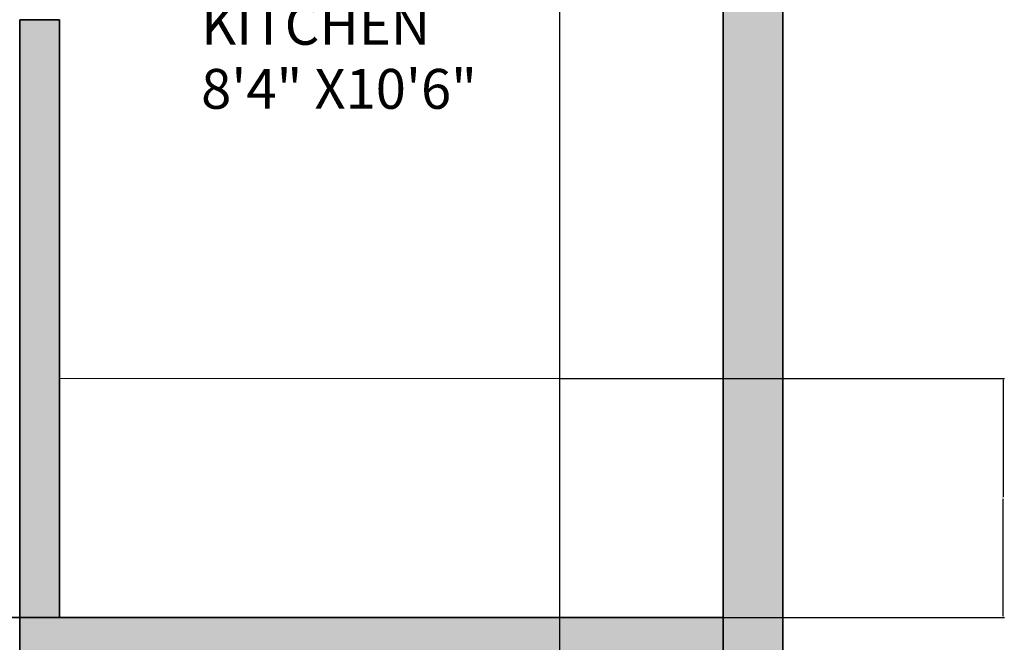
# Model space of a CAD drawing. Units: inches. Extents: x 2070 to 4408, y 1595 to 4269.
# Tile 17 of 20: x 2340 to 2489, y 2083 to 2176. Entities that reach past the tile are written whole.
import ezdxf

# ---------------------------------------------------------------- set-up
doc = ezdxf.new("R2010")
doc.units = ezdxf.units.IN
for name, color, linetype, lineweight in [('A-ANNO-DIMS', 2, 'Continuous', 18), ('A-AREA-IDEN', 7, 'Continuous', 18), ('A-FLOR-CASE', 8, 'Continuous', 18), ('A-WALL', 7, 'Continuous', 35)]:
    doc.layers.add(name, color=color, linetype=linetype, lineweight=lineweight)
doc.layers.add('A-WALL-PATT', color=18, linetype='Continuous', lineweight=13, true_color=0x000000)
doc.styles.get("Standard").update_dxf_attribs({"font": 'arial.ttf'})
doc.dimstyles.get("Standard").update_dxf_attribs({"dimtxt": 0.18, "dimasz": 0.18, "dimexe": 0.18, "dimexo": 0.0625, "dimgap": 0.09, "dimtad": 0, "dimtih": 1, "dimtoh": 1, "dimdec": 4, "dimzin": 0, "dimdsep": 46, "dimtxsty": 'Standard', "dimcen": 0.09, "dimadec": 0, "dimazin": 0, "dimtfac": 1, "dimtdec": 4, "dimtofl": 0, "dimtmove": 0, "dimatfit": 3, "dimfxl": 1, "dimtolj": 1, "dimtzin": 0, "dimarcsym": 0})

# ---------------------------------------------------------------- blocks, each defined once
blk = doc.blocks.new('*D34')
at = {"layer": 'A-ANNO-DIMS', "color": 0, "lineweight": -2, "transparency": 16777216}
for p, q in [((2421.53, 2212.34), (2421.53, 1595.04)), ((2446.2, 2212.34), (2446.2, 1595.04)), ((2421.71, 1595.22), (2433.4, 1595.22)), ((2446.02, 1595.22), (2434.33, 1595.22))]:
    blk.add_line(p, q, dxfattribs=at)
at = {"layer": 'A-ANNO-DIMS', "color": 0, "transparency": 16777216}
for points in [[(2421.71, 1595.25), (2421.71, 1595.19), (2421.53, 1595.22)], [(2446.02, 1595.25), (2446.02, 1595.19), (2446.2, 1595.22)]]:
    blk.add_solid(points, dxfattribs=at)
at = {"layer": 'Defpoints', "color": 0, "transparency": 16777216}
for p in [(2421.53, 2212.4), (2446.2, 2212.4), (2446.2, 1595.22)]:
    blk.add_point(p, dxfattribs=at)
at = {"layer": 'A-ANNO-DIMS', "color": 0, "transparency": 16777216, "insert": (2433.86, 1595.22), "char_height": 0.18, "attachment_point": 5}
blk.add_mtext('\\A1;24.663', dxfattribs=at)
blk = doc.blocks.new('*D35')
at = {"layer": 'A-ANNO-DIMS', "color": 0, "lineweight": -2, "transparency": 16777216}
for p, q in [((2421.6, 2122.4), (2488.56, 2122.4)), ((2488.38, 2122.22), (2488.38, 2104.58)), ((2488.38, 2086.58), (2488.38, 2104.22)), ((2446.26, 2086.4), (2488.56, 2086.4))]:
    blk.add_line(p, q, dxfattribs=at)
at = {"layer": 'A-ANNO-DIMS', "color": 0, "transparency": 16777216}
for points in [[(2488.35, 2122.22), (2488.41, 2122.22), (2488.38, 2122.4)], [(2488.35, 2086.58), (2488.41, 2086.58), (2488.38, 2086.4)]]:
    blk.add_solid(points, dxfattribs=at)
at = {"layer": 'Defpoints', "color": 0, "transparency": 16777216}
for p in [(2421.53, 2122.4), (2446.2, 2086.4), (2488.38, 2086.4)]:
    blk.add_point(p, dxfattribs=at)
at = {"layer": 'A-ANNO-DIMS', "color": 0, "transparency": 16777216, "insert": (2488.38, 2104.4), "char_height": 0.18, "attachment_point": 5}
blk.add_mtext('\\A1;36', dxfattribs=at)

msp = doc.modelspace()

# ---------------------------------------------------------------- hatches: boundary and pattern name
at = {"layer": 'A-WALL-PATT'}
h = msp.add_hatch(color=256, dxfattribs=at)
h.dxf.hatch_style = 1
h.paths.add_polyline_path([(2346.196, 2218.3995), (2346.196, 2282.3995), (2340.196, 2282.3995), (2340.196, 2212.3995), (2345.5866, 2212.3995), (2346.196, 2212.3995)], flags=0)
h.paths.add_polyline_path([(2245.196, 2282.3995), (2239.196, 2282.3995), (2239.196, 2186.3995), (2244.5866, 2186.3995), (2245.196, 2186.3995)], flags=0)
h.paths.add_polyline_path([(2340.196, 2230.6455), (2245.196, 2230.6455), (2245.196, 2224.6455), (2340.196, 2224.6455)], flags=0)
h.paths.add_polyline_path([(2245.196, 2150.3995), (2239.196, 2150.3995), (2164.4362, 2150.3995), (2164.4362, 2144.3995), (2239.196, 2144.3995), (2239.196, 2086.3995), (2239.196, 2067.2711), (2244.5866, 2067.2711), (2245.196, 2067.2711), (2245.196, 2144.3995)], flags=0)
h.paths.add_polyline_path([(2346.196, 2176.3995), (2340.196, 2176.3995), (2340.196, 2086.3995), (2346.196, 2086.3995), (2346.196, 2125.318)], flags=0)
h.paths.add_polyline_path([(2446.196, 2086.3995), (2346.196, 2086.3995), (2340.196, 2086.3995), (2340.196, 2080.3995), (2446.196, 2080.3995)], flags=0)
h.paths.add_polyline_path([(2455.196, 2291.3995), (2103.196, 2291.3995), (2103.196, 1699.3995), (2336.196, 1699.3995), (2336.196, 1628.3995), (2345.196, 1628.3995), (2446.196, 1628.3995), (2454.8846, 1628.3995), (2454.8846, 1699.3995)])
h.paths.add_polyline_path([(2446.196, 2282.3995), (2446.196, 2218.3995), (2446.196, 2212.3995), (2446.196, 2086.3995), (2446.196, 2080.3995), (2446.196, 1708.3995), (2446.196, 1637.3995), (2345.196, 1637.3995), (2345.196, 1699.3995), (2345.196, 1708.3995), (2336.196, 1708.3995), (2112.196, 1708.3995), (2112.196, 2282.3995), (2239.196, 2282.3995), (2245.196, 2282.3995), (2356.196, 2282.3995)], flags=16)
h.paths.add_polyline_path([(2245.196, 2150.3995), (2245.196, 2144.3995), (2245.196, 2067.2711), (2244.5866, 2067.2711), (2239.196, 2067.2711), (2239.196, 2065.6988), (2203.2929, 2065.6988, 0.40145271), (2239.196, 2031.3337), (2244.5866, 2031.3337), (2245.196, 2031.2711), (2245.196, 1924.1525), (2239.196, 1924.1525), (2239.196, 1922.5803), (2203.2929, 1922.5803, 0.40145271), (2239.196, 1888.2151), (2244.5866, 1888.2151), (2245.196, 1888.1525), (2245.196, 1748.3995), (2339.196, 1748.4621, -0.40145271), (2303.2929, 1782.8272), (2303.2585, 1782.8272), (2303.2585, 1784.3995), (2339.196, 1784.3995), (2339.196, 1877.2067), (2291.196, 1877.2067), (2291.196, 1883.2067), (2291.196, 1946.3995), (2291.196, 1952.3995), (2291.196, 2086.3995), (2297.196, 2086.3995), (2302.196, 2086.3995), (2302.196, 2081.0259), (2303.7633, 2081.0259), (2303.7633, 2080.3995), (2338.0148, 2080.3995, 0.00437129), (2338.0203, 2081.0259), (2338.0203, 2086.3995), (2340.196, 2086.3995), (2340.196, 2176.4621), (2345.5866, 2176.4621, 0.40145271), (2381.4896, 2210.8272), (2345.5866, 2210.8272), (2345.5866, 2212.3995), (2340.196, 2212.3995), (2340.196, 2224.6455), (2245.196, 2224.6455), (2245.196, 2186.3995), (2244.5866, 2186.3995), (2239.196, 2186.3995), (2239.196, 2184.8272), (2203.2929, 2184.8272, 0.40145271), (2239.196, 2150.4621), (2244.5866, 2150.4621)], flags=0)
h.paths.add_polyline_path([(2346.196, 2282.3995), (2346.196, 2218.3995), (2377.1813, 2218.3995), (2377.1813, 2212.3995), (2346.196, 2212.3995), (2345.5866, 2212.3995), (2340.196, 2212.3995), (2340.196, 2224.6455), (2245.196, 2224.6455), (2245.196, 2230.6455), (2245.196, 2282.3995), (2292.696, 2256.5225), (2340.196, 2282.3995)], flags=0)
h.paths.add_polyline_path([(2346.196, 2086.3995), (2340.196, 2086.3995), (2340.196, 2080.3995), (2446.196, 2080.3995), (2431.196, 2016.3995), (2446.196, 1952.3995), (2412.196, 1952.3995), (2412.196, 2080.3995), (2340.196, 2080.3995), (2340.196, 2086.3995), (2340.196, 2176.3995), (2346.196, 2176.3995), (2346.196, 2125.318)], flags=0)
h.paths.add_polyline_path([(2186.508, 2270.0471, -0.03755288), (2186.9712, 2269.8581), (2186.9164, 2270.112, -0.02759121)], flags=0)
h.paths.add_polyline_path([(2183.955, 2273.7766, 1), (2188.2945, 2273.7766, 1)], flags=0)
h.paths.add_polyline_path([(2142.5261, 2274.6158, -0.03707541), (2142.5672, 2275.1696), (2142.5672, 2276.826), (2119.8759, 2276.826), (2119.8759, 2263.0962), (2140.4332, 2263.0962), (2142.5672, 2263.0962), (2142.5672, 2274.0621, -0.03707541)], flags=0)
h.paths.add_polyline_path([(2209.8974, 2263.0962), (2209.8974, 2262.2079), (2190.8042, 2262.2079), (2190.8042, 2263.0962)], flags=0)
h.paths.add_polyline_path([(2210.6382, 2276.1833), (2210.6382, 2263.9844), (2190.2185, 2263.9844), (2190.2185, 2276.1833)], flags=0)
h.paths.add_polyline_path([(2188.4362, 2273.7766, -1), (2183.8133, 2273.7766, -1)], flags=0)
h.paths.add_polyline_path([(2245.196, 2150.3995), (2245.196, 2144.3995), (2245.196, 2067.2711), (2239.196, 2067.2711), (2239.196, 2080.3995), (2172.196, 2080.3995), (2172.196, 2000.3995), (2239.196, 2000.3995), (2239.196, 1940.3995), (2159.0187, 1940.3995), (2123.0187, 1940.3995), (2112.196, 1940.3995), (2112.196, 1946.3995), (2123.0187, 1946.3995), (2123.0187, 1982.2238), (2124.586, 1982.2238), (2124.586, 1982.1895, -0.40145271), (2158.8429, 1946.3995), (2159.0187, 1946.3995), (2239.196, 1946.3995), (2239.196, 1994.3995), (2112.196, 1994.3995), (2112.196, 2000.3995), (2139.196, 2040.3995), (2112.196, 2080.3995), (2112.196, 2086.3995), (2239.196, 2086.3995), (2239.196, 2144.3995), (2209.5809, 2144.3995), (2209.5809, 2136.3995), (2203.0809, 2136.3995), (2205.0809, 2130.3996, -0.70257121), (2199.081, 2116.3995, -0.70256205), (2193.0809, 2130.3994), (2195.0809, 2136.3995), (2192.0809, 2136.3995), (2192.0809, 2134.8995), (2189.0809, 2134.8995), (2189.0809, 2135.8995), (2191.0809, 2135.8995), (2191.0809, 2136.3995), (2188.5809, 2136.3995), (2188.5809, 2144.3995), (2164.2481, 2144.3995, -0.39385849), (2130.0035, 2109.5491), (2130.0035, 2109.5147), (2128.4362, 2109.5147), (2128.4362, 2144.3995), (2112.196, 2144.3995), (2112.196, 2150.3995), (2128.4362, 2150.3995), (2128.4362, 2150.7127), (2164.4362, 2150.7127), (2164.4362, 2150.3995), (2239.196, 2150.3995)], flags=0)
h.paths.add_polyline_path([(2188.2075, 2266.8735), (2188.2075, 2211.8632, -0.41421356), (2185.4833, 2209.1391), (2146.7995, 2209.1391, -0.41421356), (2144.0754, 2211.8632), (2144.0754, 2266.8735, -0.41421356), (2146.7995, 2269.5976), (2185.4833, 2269.5976, -0.41421356)], flags=0)
h.paths.add_polyline_path([(2185.0844, 2273.7766, -1), (2187.1651, 2273.7766, -1)], flags=0)
h.paths.add_polyline_path([(2182.0486, 2259.2932), (2168.0953, 2259.2932), (2168.0953, 2260.8424), (2163.7261, 2260.8424), (2163.7261, 2259.2932), (2149.7727, 2259.2932), (2149.7727, 2266.3352), (2163.7261, 2266.3352), (2163.7261, 2261.9839), (2168.0953, 2261.9839), (2168.0953, 2266.3352), (2182.0486, 2266.3352)], flags=0)
h.paths.add_polyline_path([(2148.2585, 2250.2051), (2153.0615, 2241.8861, 0.39807048)], flags=0)
h.paths.add_polyline_path([(2162.7572, 2247.2885), (2153.1461, 2241.7396), (2148.1083, 2250.4653), (2157.7194, 2256.0142)], flags=0)
h.paths.add_polyline_path([(2162.6726, 2247.4351, -0.39286196), (2157.8415, 2255.6313), (2157.6431, 2255.6313), (2157.8696, 2255.7541)], flags=0)
h.paths.add_polyline_path([(2164.2604, 2145.339), (2164.4362, 2144.3995), (2164.4362, 2150.3995), (2164.2604, 2150.7127)], flags=0)
h.paths.add_polyline_path([(2208.5809, 2142.6495), (2208.5809, 2138.3995, -0.41421356), (2207.8309, 2137.3995), (2190.5809, 2137.3995, -0.41421356), (2189.5809, 2138.1495), (2189.5809, 2142.3995, -0.41421356), (2190.3309, 2143.3995), (2207.5809, 2143.3995, -0.41421356)], flags=0)
h.paths.add_polyline_path([(2147.957, 2229.9119), (2154.7494, 2223.1195, 0.39807048)], flags=0)
h.paths.add_polyline_path([(2162.7165, 2230.8473), (2154.8691, 2222.9998), (2147.7446, 2230.1244), (2155.592, 2237.9718)], flags=0)
h.paths.add_polyline_path([(2162.5969, 2230.9669, -0.39807048), (2155.8044, 2237.7594)], flags=0)
h.paths.add_polyline_path([(2391.8776, 2049.9192), (2408.5766, 2049.9192), (2408.5766, 2033.2202), (2408.5766, 1983.123), (2408.5766, 1966.4239), (2391.8776, 1966.4239), (2391.8776, 1983.123), (2341.7804, 1983.123), (2341.7804, 2033.2202), (2391.8776, 2033.2202)], flags=0)
h.paths.add_polyline_path([(2144.1055, 2274.6158, 1), (2148.445, 2274.6158, 1)], flags=0)
h.paths.add_polyline_path([(2148.5867, 2274.6158, -1), (2143.9638, 2274.6158, -1)], flags=0)
h.paths.add_polyline_path([(2145.2349, 2274.6158, -1), (2147.3156, 2274.6158, -1)], flags=0)
edge = h.paths.add_edge_path(flags=0)
edge.add_ellipse((2400.5951, 2040.9436), major_axis=(-4.5109, 0), ratio=0.97544784, start_angle=180, end_angle=270, ccw=False)
edge.add_ellipse((2400.5951, 2040.9436), major_axis=(-4.5109, 0), ratio=0.97544784, start_angle=90, end_angle=180, ccw=False)
edge.add_ellipse((2400.5951, 2040.9436), major_axis=(-4.5109, 0), ratio=0.97544784, start_angle=0, end_angle=90, ccw=False)
edge.add_ellipse((2400.5951, 2040.9436), major_axis=(-4.5109, 0), ratio=0.97544784, start_angle=270, end_angle=360, ccw=False)
h.paths.add_polyline_path([(2199.0809, 2117.3995, -0.73452973), (2195.0809, 2130.3995), (2203.081, 2130.3995, -0.73453329)], flags=0)
h.paths.add_polyline_path([(2141.9147, 2276.0353), (2141.9147, 2263.9844), (2120.4685, 2263.9844), (2120.4685, 2276.0353)], flags=0)
h.paths.add_polyline_path([(2138.4481, 2273.4072), (2138.4481, 2266.7226), (2133.2801, 2266.7226), (2133.2801, 2273.4072)], flags=0)
h.paths.add_polyline_path([(2137.9691, 2272.9175), (2137.9691, 2272.204), (2135.4229, 2272.204), (2135.4229, 2271.6329), (2135.3221, 2270.1051), (2135.3221, 2269.0265), (2135.4229, 2268.6811), (2135.4229, 2267.2011), (2133.7212, 2267.2011), (2133.7212, 2268.6811), (2133.7983, 2269.9587), (2133.7983, 2271.2758), (2133.7212, 2271.6329), (2133.7212, 2273.0065), (2135.717, 2273.0065), (2135.717, 2272.9175)], flags=0)
h.paths.add_polyline_path([(2137.9215, 2271.8264), (2137.9215, 2271.3786), (2137.5182, 2271.3786), (2136.9355, 2271.3786), (2136.3529, 2271.3786), (2135.7703, 2271.3786), (2135.7703, 2271.8264), (2136.1736, 2271.8264), (2136.7562, 2271.8264), (2137.3389, 2271.8264)], flags=0)
h.paths.add_polyline_path([(2137.9215, 2271.692), (2137.5182, 2271.692), (2136.9355, 2271.513), (2137.3389, 2271.513)], flags=0)
h.paths.add_polyline_path([(2136.3529, 2271.692), (2135.7703, 2271.513), (2136.1736, 2271.513), (2136.7562, 2271.692)], flags=0)
h.paths.add_polyline_path([(2137.9215, 2271.513), (2137.5182, 2271.513), (2136.7562, 2271.747), (2136.7562, 2271.692), (2137.3389, 2271.692)], flags=0)
h.paths.add_polyline_path([(2137.8207, 2270.4664), (2137.8207, 2270.0971), (2137.8207, 2269.627), (2137.8207, 2269.1569), (2137.8207, 2268.6868), (2137.3837, 2268.6868), (2136.6442, 2268.6868), (2135.9271, 2268.6868), (2135.9271, 2269.0562), (2135.9271, 2269.5263), (2135.9271, 2269.9963), (2135.9271, 2270.4664), (2136.3641, 2270.4664), (2137.0812, 2270.4664)], flags=0)
h.paths.add_polyline_path([(2137.3837, 2269.627), (2137.8207, 2269.627), (2137.8207, 2269.5263), (2137.3837, 2269.5263), (2137.3837, 2269.1569), (2137.8207, 2269.1569), (2137.3837, 2269.0562), (2137.3837, 2268.6868), (2137.0812, 2268.6868), (2137.0812, 2269.0562), (2136.6442, 2269.0562), (2136.6442, 2268.6868), (2136.3641, 2268.6868), (2136.3641, 2269.0562), (2135.9271, 2269.0562), (2135.9271, 2269.1569), (2136.3641, 2269.1569), (2136.3641, 2269.5263), (2135.9271, 2269.5263), (2135.9271, 2269.627), (2136.3641, 2269.627), (2136.3641, 2269.9963), (2135.9271, 2269.9963), (2136.3641, 2270.0971), (2136.3641, 2270.4664), (2136.6442, 2270.4664), (2136.6442, 2270.0971), (2137.0812, 2270.0971), (2137.0812, 2270.4664), (2137.3837, 2270.4664), (2137.3837, 2270.0971), (2137.8207, 2270.0971), (2137.3837, 2269.9963)], flags=0)
h.paths.add_polyline_path([(2137.5182, 2271.8264), (2137.5182, 2271.692), (2137.3389, 2271.3786), (2137.3389, 2271.513)], flags=0)
h.paths.add_polyline_path([(2137.8179, 2267.8138), (2137.8179, 2267.6879), (2137.1876, 2267.6879), (2136.4733, 2267.6879), (2135.759, 2267.6879), (2135.759, 2267.8138), (2136.3893, 2267.8138), (2137.1036, 2267.8138)], flags=0)
h.paths.add_polyline_path([(2137.0812, 2269.9963), (2137.0812, 2269.627), (2137.0812, 2269.1569), (2136.6442, 2269.1569), (2136.6442, 2269.5263), (2136.6442, 2269.9963)], flags=0)
h.paths.add_polyline_path([(2136.3529, 2271.8264), (2136.3529, 2271.692), (2136.1736, 2271.3786), (2136.1736, 2271.513)], flags=0)
h.paths.add_polyline_path([(2136.4733, 2267.8138), (2136.4733, 2267.6879), (2136.3893, 2267.6879), (2136.3893, 2267.8138)], flags=0)
h.paths.add_polyline_path([(2407.9087, 2032.5522), (2407.9087, 1983.7909), (2359.81, 1983.7909, -0.00912788), (2359.0575, 1983.7909), (2342.4483, 1983.7909), (2342.4483, 2032.5522)], flags=0)
h.paths.add_polyline_path([(2389.1838, 2023.1358), (2353.7856, 2023.1358), (2353.7856, 1985.4867, -0.09210376), (2350.2788, 1988.655), (2350.2788, 2026.6426), (2389.1838, 2026.6426)], flags=0)
h.paths.add_polyline_path([(2352.6166, 2024.3048), (2351.4477, 2024.3048), (2351.4477, 2025.4737), (2352.6166, 2025.4737)], flags=0)
h.paths.add_polyline_path([(2399.6319, 2026.7589), (2404.3661, 2026.7589, -0.41421356), (2407.0379, 2024.087), (2407.0379, 2013.4908, -0.41421356), (2404.3661, 2010.819), (2399.6319, 2010.819, -0.41421356), (2396.96, 2013.4908), (2396.96, 2024.087, -0.41421356)], flags=0)
h.paths.add_polyline_path([(2399.6319, 2026.0909), (2404.3661, 2026.0909, -0.41421356), (2406.37, 2024.087), (2406.37, 2013.4908, -0.41421356), (2404.3661, 2011.487), (2399.6319, 2011.487, -0.41421356), (2397.628, 2013.4908), (2397.628, 2024.087, -0.41421356)], flags=0)
h.paths.add_polyline_path([(2399.6319, 2002.3217), (2404.3661, 2002.3217, -0.41421356), (2407.0379, 1999.6498), (2407.0379, 1989.0536, -0.41421356), (2404.3661, 1986.3818), (2399.6319, 1986.3818, -0.41421356), (2396.96, 1989.0536), (2396.96, 1999.6498, -0.41421356)], flags=0)
h.paths.add_polyline_path([(2399.6319, 2001.6537), (2404.3661, 2001.6537, -0.41421356), (2406.37, 1999.6498), (2406.37, 1989.0536, -0.41421356), (2404.3661, 1987.0497), (2399.6319, 1987.0497, -0.41421356), (2397.628, 1989.0536), (2397.628, 1999.6498, -0.41421356)], flags=0)
edge = h.paths.add_edge_path(flags=0)
edge.add_ellipse((2400.5951, 1975.3996), major_axis=(-4.5109, 0), ratio=0.97544784, start_angle=-180, end_angle=-90, ccw=False)
edge.add_ellipse((2400.5951, 1975.3996), major_axis=(-4.5109, 0), ratio=0.97544784, start_angle=90, end_angle=180, ccw=False)
edge.add_ellipse((2400.5951, 1975.3996), major_axis=(-4.5109, 0), ratio=0.97544784, start_angle=0, end_angle=90, ccw=False)
edge.add_ellipse((2400.5951, 1975.3996), major_axis=(-4.5109, 0), ratio=0.97544784, start_angle=-90, end_angle=0, ccw=False)
h.paths.add_polyline_path([(2345.196, 1910.3995), (2366.4386, 1910.3995), (2366.4386, 1925.4555), (2392.3856, 1925.4555), (2392.3856, 1933.5025), (2400.1399, 1925.4555), (2392.3856, 1919.8795), (2392.3856, 1925.4555), (2366.4386, 1925.4555), (2366.4386, 1910.3995), (2381.196, 1910.3995), (2405.196, 1910.3995), (2405.196, 1898.3995), (2446.196, 1898.3995), (2446.196, 1886.3995), (2405.196, 1886.3995), (2405.196, 1874.3995), (2446.196, 1874.3995), (2446.196, 1862.3995), (2405.196, 1862.3995), (2405.196, 1850.3995), (2446.196, 1850.3995), (2446.196, 1838.3995), (2405.196, 1838.3995), (2405.196, 1826.3995), (2446.196, 1826.3995), (2446.196, 1814.3995), (2405.196, 1814.3995), (2405.196, 1802.3995), (2446.196, 1802.3995), (2446.196, 1798.3995), (2446.196, 1792.3995), (2405.196, 1792.3995), (2405.196, 1910.3995), (2381.196, 1910.3995), (2381.196, 1792.3995), (2345.196, 1792.3995)], flags=0)
h.paths.add_polyline_path([(2333.0944, 1863.3993, -0.41421356), (2334.7225, 1861.7712), (2334.7225, 1859.329), (2335.2653, 1859.329, -0.41421356), (2337.4361, 1857.1582), (2337.4361, 1843.862, -0.41421356), (2335.2653, 1841.6911, -0.41421356), (2337.4361, 1839.5203), (2337.4361, 1827.5808, -0.41421356), (2335.2653, 1825.41, -0.41421356), (2337.4361, 1823.2392), (2337.4361, 1808.5862, -0.41421356), (2335.2653, 1806.4153), (2334.7225, 1806.4153), (2334.7225, 1803.9732, -0.41421356), (2333.0944, 1802.3451), (2317.356, 1802.3451), (2317.0846, 1802.3451, -0.41421356), (2315.7279, 1803.7018), (2315.7279, 1803.8646), (2313.8284, 1803.8646, -0.41421356), (2311.6576, 1806.0354), (2311.6576, 1823.2015, -0.39597602), (2313.6834, 1825.3765, -0.43384798), (2311.6576, 1827.2718), (2311.6576, 1839.761, -0.41421356), (2313.5571, 1841.6604), (2313.8284, 1841.6604), (2333.8159, 1841.6604, -0.04213623), (2334.1798, 1841.6911, -0.41421356), (2332.009, 1843.862), (2332.009, 1857.1582, -0.41421356), (2334.1798, 1859.329), (2317.356, 1859.329), (2317.0846, 1859.329, -0.41421356), (2315.7279, 1860.6858), (2315.7279, 1862.0426, -0.41421356), (2317.0846, 1863.3993), (2317.356, 1863.3993)], flags=0)
h.paths.add_polyline_path([(2208.8475, 1848.9818), (2208.8475, 1840.9741, -0.41421356), (2207.0458, 1839.1724), (2206.5453, 1839.1721), (2206.5453, 1838.7218, -0.40985861), (2204.7704, 1836.9203), (2183.7501, 1836.9203, -0.41858196), (2181.9216, 1838.7218), (2181.9216, 1839.1721), (2181.421, 1839.1724, -0.41421356), (2179.6193, 1840.9741), (2179.6193, 1848.6817, -0.44064415), (2185.1126, 1854.9874), (2203.3852, 1854.9874, -0.45707961)], flags=0)
h.paths.add_polyline_path([(2204.243, 1848.4815), (2204.243, 1848.4815, 0.41725335), (2202.2204, 1850.4833), (2186.2049, 1850.4833, 0.4111805), (2184.2237, 1848.4815), (2184.2237, 1848.4815, -0.4111807), (2186.2049, 1850.4833), (2202.2204, 1850.4833, -0.41725315)], flags=0)
h.paths.add_polyline_path([(2234.7177, 1830.228), (2234.7176, 1781.6047, -0.41421356), (2233.4381, 1780.3252), (2218.6064, 1780.3252, -0.41421356), (2217.8387, 1781.0929), (2217.8387, 1783.3961, -0.41421356), (2218.6064, 1784.1639), (2218.6065, 1796.9595, -0.41421356), (2219.886, 1798.239, -0.41421356), (2218.6065, 1799.5186), (2218.6065, 1812.3142, -0.41421356), (2219.8861, 1813.5938, -0.41421356), (2218.6065, 1814.8733), (2218.6065, 1827.6689, -0.41421356), (2217.8388, 1828.4367), (2217.8388, 1830.7399, -0.41421356), (2218.6065, 1831.5076), (2233.4382, 1831.5076, -0.41421356)], flags=0)
h.paths.add_polyline_path([(2230.6344, 1827.6689, -0.41421356), (2231.4021, 1826.9012), (2231.4021, 1784.9316, -0.41421356), (2230.6343, 1784.1639), (2221.1853, 1784.1639), (2221.1853, 1827.6689)], flags=0)
h.paths.add_polyline_path([(2222.7208, 1798.239), (2221.6971, 1798.239), (2221.6971, 1813.5938), (2222.7208, 1813.5938)], flags=0)
h.paths.add_polyline_path([(2206.5453, 1773.935), (2206.5453, 1773.4848), (2206.9457, 1773.4848), (2207.0458, 1773.4845, -0.41421356), (2208.8475, 1771.6827), (2208.8475, 1763.675, -0.44222432), (2203.6505, 1757.6695), (2185.3851, 1757.6695, -0.45508402), (2179.6193, 1763.9752), (2179.6193, 1771.6827, -0.41421356), (2181.421, 1773.4845), (2181.421, 1773.4848), (2181.9216, 1773.4848), (2181.9216, 1773.935, -0.40985861), (2183.6965, 1775.7366), (2204.7167, 1775.7366, -0.41858196)], flags=0)
h.paths.add_polyline_path([(2202.2619, 1762.1736), (2186.2464, 1762.1736, -0.41725315), (2184.2237, 1764.1754), (2184.2237, 1764.1754, 0.41725335), (2186.2464, 1762.1736), (2202.2619, 1762.1736, 0.4111805), (2204.243, 1764.1754), (2204.243, 1764.1754, -0.4111807)], flags=0)
h.paths.add_polyline_path([(2313.0034, 1713.1906), (2312.997, 1713.1697), (2313.0123, 1713.1612)], flags=0)
h.paths.add_polyline_path([(2305.7314, 1721.0488), (2305.6257, 1721.1994), (2305.4853, 1721.084)], flags=0)
h.paths.add_polyline_path([(2307.5562, 1726.1427), (2307.6186, 1726.1026), (2307.5737, 1726.0477), (2308.5692, 1720.6434), (2310.5345, 1721.2985), (2310.5721, 1721.411), (2310.6958, 1721.3523), (2313.8453, 1722.4021), (2314.9351, 1723.8033), (2314.9294, 1723.9165), (2315.0028, 1723.8903), (2313.874, 1722.4389), (2313.8697, 1722.4102), (2308.5692, 1720.6434), (2308.9864, 1720.122), (2309.0665, 1720.0971), (2309.053, 1720.0387), (2310.9235, 1717.7005), (2311.4182, 1717.6259), (2311.2918, 1717.2402), (2312.0655, 1716.2731), (2312.1081, 1716.2606), (2312.0969, 1716.2339), (2308.5692, 1720.6434), (2305.2249, 1717.745), (2305.232, 1717.704), (2305.1665, 1717.6944), (2308.5692, 1720.6434)], flags=0)
h.paths.add_polyline_path([(2288.2072, 1714.3431), (2288.2008, 1714.3222), (2288.216, 1714.3137)], flags=0)
h.paths.add_polyline_path([(2280.9352, 1722.2013), (2280.8295, 1722.3519), (2280.689, 1722.2365)], flags=0)
h.paths.add_polyline_path([(2282.76, 1727.2952), (2282.8224, 1727.2551), (2282.7775, 1727.2002), (2283.773, 1721.7959), (2285.7383, 1722.451), (2285.7759, 1722.5635), (2285.8995, 1722.5048), (2289.0491, 1723.5546), (2290.1389, 1724.9558), (2290.1332, 1725.069), (2290.2065, 1725.0428), (2289.0777, 1723.5915), (2289.0735, 1723.5628), (2283.773, 1721.7959), (2284.1901, 1721.2745), (2284.2703, 1721.2496), (2284.2567, 1721.1913), (2286.1273, 1718.8531), (2286.622, 1718.7785), (2286.4956, 1718.3927), (2287.2692, 1717.4256), (2287.3119, 1717.4131), (2287.3006, 1717.3864), (2283.773, 1721.7959), (2280.4286, 1718.8975), (2280.4357, 1718.8565), (2280.3703, 1718.8469), (2283.773, 1721.7959)], flags=0)
h.paths.add_polyline_path([(2302.0672, 1721.8694), (2301.8205, 1721.8572), (2301.7578, 1722.1787), (2299.415, 1724.5215), (2299.103, 1724.4694), (2299.0662, 1724.8703)], flags=0)
h.paths.add_polyline_path([(2264.5643, 1715.4956), (2264.5579, 1715.4747), (2264.5731, 1715.4662)], flags=0)
h.paths.add_polyline_path([(2257.2923, 1723.3538), (2257.1865, 1723.5044), (2257.0461, 1723.389)], flags=0)
h.paths.add_polyline_path([(2259.117, 1728.4477), (2259.1795, 1728.4077), (2259.1345, 1728.3527), (2260.13, 1722.9484), (2262.0954, 1723.6036), (2262.133, 1723.716), (2262.2566, 1723.6573), (2265.4061, 1724.7071), (2266.4959, 1726.1083), (2266.4902, 1726.2215), (2266.5636, 1726.1953), (2265.4348, 1724.744), (2265.4305, 1724.7153), (2260.13, 1722.9484), (2260.5472, 1722.427), (2260.6273, 1722.4022), (2260.6138, 1722.3438), (2262.4843, 1720.0056), (2262.979, 1719.931), (2262.8526, 1719.5452), (2263.6263, 1718.5781), (2263.6689, 1718.5656), (2263.6577, 1718.5389), (2260.13, 1722.9484), (2256.7857, 1720.05), (2256.7928, 1720.009), (2256.7273, 1719.9994), (2260.13, 1722.9484)], flags=0)
h.paths.add_polyline_path([(2277.2709, 1723.0219), (2277.0243, 1723.0097), (2276.9616, 1723.3312), (2274.6187, 1725.6741), (2274.3067, 1725.6219), (2274.27, 1726.0228)], flags=0)
h.paths.add_polyline_path([(2253.628, 1724.1744), (2253.3814, 1724.1622), (2253.3186, 1724.4838), (2250.9758, 1726.8266), (2250.6638, 1726.7744), (2250.627, 1727.1753)], flags=0)
h.paths.add_polyline_path([(2161.9194, 1715.4956), (2161.913, 1715.4747), (2161.9282, 1715.4662)], flags=0)
h.paths.add_polyline_path([(2154.6474, 1723.3538), (2154.5416, 1723.5044), (2154.4012, 1723.389)], flags=0)
h.paths.add_polyline_path([(2162.7899, 1724.744), (2162.7856, 1724.7153), (2157.4851, 1722.9484), (2157.9023, 1722.427), (2157.9824, 1722.4022), (2157.9689, 1722.3438), (2159.8394, 1720.0056), (2160.3341, 1719.931), (2160.2078, 1719.5452), (2160.9814, 1718.5781), (2161.024, 1718.5656), (2161.0128, 1718.5389), (2157.4851, 1722.9484), (2154.1408, 1720.05), (2154.1479, 1720.009), (2154.0824, 1719.9994), (2157.4851, 1722.9484), (2156.4721, 1728.4477), (2156.5346, 1728.4077), (2156.4896, 1728.3527), (2157.4851, 1722.9484), (2159.4505, 1723.6036), (2159.4881, 1723.716), (2159.6117, 1723.6573), (2162.7612, 1724.7071), (2163.851, 1726.1083), (2163.8453, 1726.2215), (2163.9187, 1726.1953)], flags=0)
h.paths.add_polyline_path([(2150.9831, 1724.1744), (2150.7365, 1724.1622), (2150.6738, 1724.4838), (2148.3309, 1726.8266), (2148.0189, 1726.7744), (2147.9822, 1727.1753)], flags=0)
h.paths.add_polyline_path([(2132.5099, 1716.6482), (2132.5035, 1716.6272), (2132.5187, 1716.6187)], flags=0)
h.paths.add_polyline_path([(2125.2379, 1724.5064), (2125.1322, 1724.6569), (2124.9917, 1724.5415)], flags=0)
h.paths.add_polyline_path([(2133.3804, 1725.8965), (2133.3762, 1725.8678), (2128.0757, 1724.101), (2128.4928, 1723.5795), (2128.5729, 1723.5547), (2128.5594, 1723.4963), (2130.43, 1721.1581), (2130.9246, 1721.0835), (2130.7983, 1720.6977), (2131.5719, 1719.7306), (2131.6146, 1719.7181), (2131.6033, 1719.6914), (2128.0757, 1724.101), (2124.7313, 1721.2025), (2124.7384, 1721.1615), (2124.6729, 1721.1519), (2128.0757, 1724.101), (2127.0626, 1729.6002), (2127.1251, 1729.5602), (2127.0801, 1729.5052), (2128.0757, 1724.101), (2130.041, 1724.7561), (2130.0786, 1724.8685), (2130.2022, 1724.8098), (2133.3517, 1725.8597), (2134.4415, 1727.2608), (2134.4358, 1727.3741), (2134.5092, 1727.3478)], flags=0)
h.paths.add_polyline_path([(2121.5736, 1725.3269), (2121.327, 1725.3148), (2121.2643, 1725.6363), (2118.9214, 1727.9791), (2118.6094, 1727.9269), (2118.5727, 1728.3279)], flags=0)
h.paths.add_polyline_path([(2433.3904, 1646.406), (2433.384, 1646.3851), (2433.3992, 1646.3766)], flags=0)
h.paths.add_polyline_path([(2426.1184, 1654.2642), (2426.0127, 1654.4148), (2425.8722, 1654.2994)], flags=0)
h.paths.add_polyline_path([(2427.9432, 1659.3581), (2428.0056, 1659.318), (2427.9606, 1659.2631), (2428.9562, 1653.8588), (2430.9215, 1654.514), (2430.9591, 1654.6264), (2431.0827, 1654.5677), (2434.2323, 1655.6175), (2435.322, 1657.0187), (2435.3163, 1657.1319), (2435.3897, 1657.1057), (2434.2609, 1655.6544), (2434.2567, 1655.6257), (2428.9562, 1653.8588), (2429.3733, 1653.3374), (2429.4534, 1653.3126), (2429.4399, 1653.2542), (2431.3105, 1650.916), (2431.8051, 1650.8414), (2431.6788, 1650.4556), (2432.4524, 1649.4885), (2432.4951, 1649.476), (2432.4838, 1649.4493), (2428.9562, 1653.8588), (2425.6118, 1650.9604), (2425.6189, 1650.9194), (2425.5535, 1650.9098), (2428.9562, 1653.8588)], flags=0)
h.paths.add_polyline_path([(2376.63, 1645.4912), (2376.6236, 1645.4703), (2376.6388, 1645.4617)], flags=0)
h.paths.add_polyline_path([(2369.358, 1653.3494), (2369.2523, 1653.5), (2369.1118, 1653.3845)], flags=0)
h.paths.add_polyline_path([(2371.1828, 1658.4432), (2371.2452, 1658.4032), (2371.2003, 1658.3482), (2372.1958, 1652.944), (2374.1611, 1653.5991), (2374.1987, 1653.7116), (2374.3224, 1653.6528), (2377.4719, 1654.7027), (2378.5617, 1656.1038), (2378.556, 1656.2171), (2378.6293, 1656.1908), (2377.5005, 1654.7395), (2377.4963, 1654.7108), (2372.1958, 1652.944), (2372.6129, 1652.4225), (2372.6931, 1652.3977), (2372.6795, 1652.3393), (2374.5501, 1650.0011), (2375.0448, 1649.9265), (2374.9184, 1649.5407), (2375.692, 1648.5737), (2375.7347, 1648.5611), (2375.7234, 1648.5344), (2372.1958, 1652.944), (2368.8514, 1650.0456), (2368.8586, 1650.0046), (2368.7931, 1649.995), (2372.1958, 1652.944)], flags=0)
h.paths.add_polyline_path([(2404.0947, 1645.0338), (2404.0883, 1645.0128), (2404.1035, 1645.0043)], flags=0)
h.paths.add_polyline_path([(2396.8227, 1652.892), (2396.717, 1653.0425), (2396.5765, 1652.9271)], flags=0)
h.paths.add_polyline_path([(2398.6475, 1657.9858), (2398.7099, 1657.9458), (2398.665, 1657.8908), (2399.6605, 1652.4866), (2401.6258, 1653.1417), (2401.6634, 1653.2541), (2401.7871, 1653.1954), (2404.9366, 1654.2453), (2406.0264, 1655.6464), (2406.0207, 1655.7596), (2406.094, 1655.7334), (2404.9652, 1654.2821), (2404.961, 1654.2534), (2399.6605, 1652.4866), (2400.0776, 1651.9651), (2400.1578, 1651.9403), (2400.1442, 1651.8819), (2402.0148, 1649.5437), (2402.5095, 1649.4691), (2402.3831, 1649.0833), (2403.1567, 1648.1162), (2403.1994, 1648.1037), (2403.1881, 1648.077), (2399.6605, 1652.4866), (2396.3162, 1649.5881), (2396.3233, 1649.5471), (2396.2578, 1649.5375), (2399.6605, 1652.4866)], flags=0)
h.paths.add_polyline_path([(2419.4532, 1658.0857), (2422.4541, 1655.0848), (2422.2075, 1655.0726), (2422.1448, 1655.3941), (2419.8019, 1657.737), (2419.4899, 1657.6848)], flags=0)
h.paths.add_polyline_path([(2390.1575, 1656.7135), (2393.1584, 1653.7125), (2392.9118, 1653.7004), (2392.8491, 1654.0219), (2390.5063, 1656.3647), (2390.1943, 1656.3125)], flags=0)
h.paths.add_polyline_path([(2362.6928, 1657.1709), (2365.6937, 1654.1699), (2365.4471, 1654.1578), (2365.3844, 1654.4793), (2363.0416, 1656.8221), (2362.7295, 1656.77)], flags=0)
h.paths.add_polyline_path([(2419.9523, 2037.8601), (2440.2872, 2037.8601), (2440.2872, 2047.1732), (2419.9523, 2047.1732)], flags=8)
h.paths.add_polyline_path([(2370.186, 1698.9005), (2413.6287, 1698.9005), (2413.6287, 1708.0908), (2370.186, 1708.0908)], flags=8)
h.paths.add_polyline_path([(2370.1656, 1708.5185), (2430.0857, 1708.5185), (2430.0857, 1717.8316), (2370.1656, 1717.8316)], flags=8)
h.paths.add_polyline_path([(2254.1469, 1788.1883), (2302.2471, 1788.1883), (2302.2471, 1797.3786), (2254.1469, 1797.3786)], flags=8)
h.paths.add_polyline_path([(2254.1264, 1797.8063), (2326.1448, 1797.8063), (2326.1448, 1807.1194), (2254.1264, 1807.1194)], flags=8)
h.paths.add_polyline_path([(2300.08, 1914.5069), (2338.861, 1914.5069), (2338.861, 1923.6972), (2300.08, 1923.6972)], flags=8)
h.paths.add_polyline_path([(2300.0595, 1924.1249), (2331.5882, 1924.1249), (2331.5882, 1933.438), (2300.0595, 1933.438)], flags=8)
h.paths.add_polyline_path([(2176.6905, 1716.4567), (2224.1441, 1716.4567), (2224.1441, 1725.647), (2176.6905, 1725.647)], flags=8)
h.paths.add_polyline_path([(2176.67, 1726.0747), (2245.9176, 1726.0747), (2245.9176, 1735.3878), (2176.67, 1735.3878)], flags=8)
h.paths.add_polyline_path([(2339.997, 2039.7696), (2388.1034, 2039.7696), (2388.1034, 2048.9661), (2339.997, 2048.9661)], flags=8)
h.paths.add_polyline_path([(2339.9776, 2049.3928), (2388.7204, 2049.3928), (2388.7204, 2058.7059), (2339.9776, 2058.7059)], flags=8)
h.paths.add_polyline_path([(2366.0063, 2161.3825), (2409.449, 2161.3825), (2409.449, 2170.5728), (2366.0063, 2170.5728)], flags=8)
h.paths.add_polyline_path([(2365.9868, 2171.0016), (2405.879, 2171.0016), (2405.879, 2180.3085), (2365.9868, 2180.3085)], flags=8)
h.paths.add_polyline_path([(2366.0102, 2247.0726), (2407.12, 2247.0726), (2407.12, 2256.263), (2366.0102, 2256.263)], flags=8)
h.paths.add_polyline_path([(2365.9897, 2256.6906), (2397.9686, 2256.6906), (2397.9686, 2266.0037), (2365.9897, 2266.0037)], flags=8)
h.paths.add_polyline_path([(2271.8465, 2102.7885), (2307.6541, 2102.7885), (2307.6541, 2111.9849), (2271.8465, 2111.9849)], flags=8)
h.paths.add_polyline_path([(2271.8281, 2112.4126), (2304.2673, 2112.4126), (2304.2673, 2121.7196), (2271.8281, 2121.7196)], flags=8)
h.paths.add_polyline_path([(2141.6408, 2187.5934), (2182.108, 2187.5934), (2182.108, 2196.7837), (2141.6408, 2196.7837)], flags=8)
h.paths.add_polyline_path([(2141.6203, 2197.2114), (2190.3631, 2197.2114), (2190.3631, 2206.5245), (2141.6203, 2206.5245)], flags=8)
h.paths.add_polyline_path([(2165.7271, 2103.039), (2211.5027, 2103.039), (2211.5027, 2112.2293), (2165.7271, 2112.2293)], flags=8)
h.paths.add_polyline_path([(2165.7077, 2112.658), (2185.1033, 2112.658), (2185.1033, 2121.965), (2165.7077, 2121.965)], flags=8)
h.paths.add_polyline_path([(2174.945, 2048.0789), (2211.3973, 2048.0789), (2211.3973, 2057.2693), (2174.945, 2057.2693)], flags=8)
h.paths.add_polyline_path([(2174.9256, 2057.698), (2194.3212, 2057.698), (2194.3212, 2067.0049), (2174.9256, 2067.0049)], flags=8)
h.paths.add_polyline_path([(2164.8305, 1965.8394), (2202.9649, 1965.8394), (2202.9649, 1975.0297), (2164.8305, 1975.0297)], flags=8)
h.paths.add_polyline_path([(2164.8111, 1975.4584), (2184.2067, 1975.4584), (2184.2067, 1984.7654), (2164.8111, 1984.7654)], flags=8)
h.paths.add_polyline_path([(2133.0392, 1862.086), (2173.5065, 1862.086), (2173.5065, 1871.2763), (2133.0392, 1871.2763)], flags=8)
h.paths.add_polyline_path([(2133.0709, 1871.8585), (2157.0382, 1871.8585), (2157.0382, 1880.8585), (2133.0709, 1880.8585)], flags=8)
h.paths.add_polyline_path([(2406.4423, 1923.5541), (2418.8209, 1923.5541), (2418.8209, 1932.7199), (2406.4423, 1932.7199)], flags=8)
h = msp.add_hatch(color=256, dxfattribs=at)
h.dxf.hatch_style = 1
h.paths.add_polyline_path([(2245.196, 2282.3995), (2239.196, 2282.3995), (2239.196, 2186.3995), (2244.5866, 2186.3995), (2245.196, 2186.3995)])
h.paths.add_polyline_path([(2340.196, 2230.6455), (2245.196, 2230.6455), (2245.196, 2224.6455), (2340.196, 2224.6455)])
h.paths.add_polyline_path([(2346.196, 2282.3995), (2340.196, 2282.3995), (2340.196, 2212.3995), (2345.5866, 2212.3995), (2346.196, 2212.3995), (2346.196, 2218.3995)])
h.paths.add_polyline_path([(2245.196, 2144.3995), (2245.196, 2150.3995), (2239.196, 2150.3995), (2164.4362, 2150.3995), (2164.4362, 2144.3995), (2239.196, 2144.3995), (2239.196, 2086.3995), (2239.196, 2067.2711), (2244.5866, 2067.2711), (2245.196, 2067.2711)])
h.paths.add_polyline_path([(2128.4362, 2150.3995), (2112.196, 2150.3995), (2112.196, 2144.3995), (2128.4362, 2144.3995), (2128.4362, 2145.339)])
h.paths.add_polyline_path([(2239.196, 2086.3995), (2112.196, 2086.3995), (2112.196, 2080.3995), (2239.196, 2080.3995)])
h.paths.add_polyline_path([(2172.196, 2080.3995), (2166.196, 2080.3995), (2166.196, 2000.3995), (2172.196, 2000.3995)])
h.paths.add_polyline_path([(2239.196, 2000.3995), (2112.196, 2000.3995), (2112.196, 1994.3995), (2239.196, 1994.3995)])
h.paths.add_polyline_path([(2245.196, 2031.2711), (2239.196, 2031.2711), (2239.196, 2000.3995), (2239.196, 1940.3995), (2245.196, 1940.3995)])
h.paths.add_polyline_path([(2239.196, 1946.3995), (2159.0187, 1946.3995), (2159.0187, 1940.3995), (2239.196, 1940.3995)])
h.paths.add_polyline_path([(2123.0187, 1946.3995), (2112.196, 1946.3995), (2112.196, 1940.3995), (2123.0187, 1940.3995)])
h.paths.add_polyline_path([(2377.1813, 2218.3995), (2346.196, 2218.3995), (2346.196, 2212.3995), (2377.1813, 2212.3995)])
h.paths.add_polyline_path([(2446.196, 2218.3995), (2413.1813, 2218.3995), (2413.1813, 2212.3995), (2446.196, 2212.3995)])
h.paths.add_polyline_path([(2446.196, 2086.3995), (2346.196, 2086.3995), (2340.196, 2086.3995), (2340.196, 2080.3995), (2446.196, 2080.3995)], flags=17)
h.paths.add_polyline_path([(2346.196, 2125.318), (2346.196, 2176.3995), (2340.196, 2176.3995), (2340.196, 2086.3995), (2346.196, 2086.3995)])
h.paths.add_polyline_path([(2245.196, 1888.1525), (2239.196, 1888.1525), (2239.196, 1748.3995), (2245.196, 1748.3995)])
h.paths.add_polyline_path([(2345.196, 1748.3995), (2239.196, 1748.3995), (2112.196, 1748.3995), (2112.196, 1742.3995), (2239.196, 1742.3995), (2345.196, 1742.3995)])
h.paths.add_polyline_path([(2297.196, 2080.3995), (2297.196, 2086.3995), (2291.196, 2086.3995), (2291.196, 1952.3995), (2291.196, 1946.3995), (2339.196, 1946.3995), (2339.196, 1883.2067), (2291.196, 1883.2067), (2291.196, 1877.2067), (2339.196, 1877.2067), (2339.196, 1784.3995), (2345.196, 1784.3995), (2345.196, 1792.3995), (2345.196, 1946.3995), (2446.196, 1946.3995), (2446.196, 1952.3995), (2297.196, 1952.3995)])

# ---------------------------------------------------------------- linework, layer by layer
at = {"layer": 'A-FLOR-CASE'}
for p, q in [((2421.5333, 2212.3995), (2421.5333, 2122.3995)), ((2421.5333, 2122.3995), (2346.196, 2122.3995)), ((2446.196, 2086.3995), (2446.196, 2122.3995))]:
    msp.add_line(p, q, dxfattribs=at)
at = {"layer": 'A-WALL'}
for p, q in [((2446.196, 2212.3995), (2446.196, 2086.3995)), ((2340.196, 2176.3995), (2346.196, 2176.3995)), ((2340.196, 2176.3995), (2340.196, 2086.3995)), ((2346.196, 2176.3995), (2346.196, 2125.318)), ((2346.196, 2176.3995), (2346.196, 2176.3995)), ((2346.196, 2086.3995), (2346.196, 2125.318)), ((2338.196, 2086.3995), (2340.196, 2086.3995)), ((2340.196, 2086.3995), (2346.196, 2086.3995)), ((2340.196, 2086.3995), (2340.196, 2080.3995)), ((2446.196, 2086.3995), (2346.196, 2086.3995))]:
    msp.add_line(p, q, dxfattribs=at)
for points in [[(2336.196, 1699.3995), (2103.196, 1699.3995), (2103.196, 2291.3995), (2455.196, 2291.3995), (2455.196, 1699.3995), (2454.8846, 1699.3995)], [(2446.196, 2212.3995), (2446.196, 1708.3995)]]:
    msp.add_lwpolyline(points, dxfattribs=at)

# ---------------------------------------------------------------- texts
at = {"layer": 'A-AREA-IDEN'}
for s, p in [('KITCHEN', (2367.538, 2172.655)), ('8\'4" X10\'6"', (2367.538, 2163.0166))]:
    msp.add_text(s, height=6, dxfattribs=at).set_placement(p)

# ---------------------------------------------------------------- dimensions: what is measured, and where the dimension line sits
at = {"layer": 'A-ANNO-DIMS'}
dim = msp.add_linear_dim(base=(2446.196, 1595.2195), p1=(2421.5333, 2212.3995), p2=(2446.196, 2212.3995), dimstyle='Standard', override={"dimdec": 3, "dimlfac": 1, "dimrnd": 0, "dimzin": 0, "dimdsep": 46, "dimlunit": 2}, dxfattribs=at)
dim.commit()
dim.dimension.update_dxf_attribs({"geometry": '*D34', "text_midpoint": (2433.8646, 1595.2195)})
dim = msp.add_linear_dim(base=(2488.376, 2086.3995), p1=(2421.5333, 2122.3995), p2=(2446.196, 2086.3995), angle=90, dimstyle='Standard', override={"dimdec": 0, "dimlfac": 1, "dimrnd": 0, "dimzin": 0, "dimdsep": 46, "dimlunit": 2}, dxfattribs=at)
dim.commit()
dim.dimension.update_dxf_attribs({"geometry": '*D35', "text_midpoint": (2488.376, 2104.3995)})

doc.saveas('drawing.dxf')
